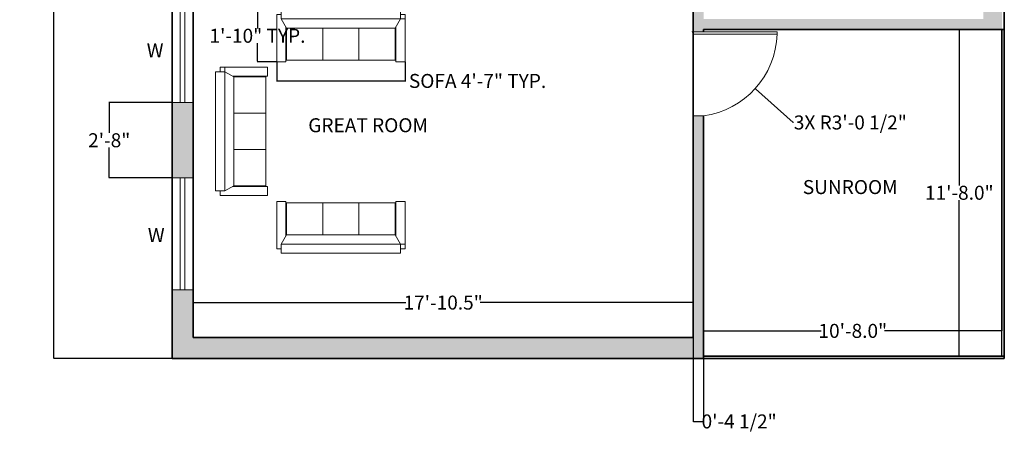
# Model space of a CAD drawing. Units: inches. Extents: x 302 to 1258, y 831 to 1373.
# Tile 7 of 13: x 781 to 1203, y 831 to 1012. Entities that reach past the tile are written whole.
import ezdxf

# ---------------------------------------------------------------- set-up
doc = ezdxf.new("R2010")
doc.units = ezdxf.units.IN
doc.header["$MEASUREMENT"] = 0
for name, color, linetype, lineweight in [('A-ANNO-DIMS', 2, 'Continuous', 18), ('A-ANNO-TEXT', 7, 'Continuous', 18), ('A-AREA-IDEN', 7, 'Continuous', 18), ('A-DOOR', 3, 'Continuous', 18), ('A-FURN', 8, 'Continuous', 18), ('A-GLAZ', 4, 'Continuous', 18), ('A-WALL', 7, 'Continuous', 35), ('A-WALL-PATT', 251, 'Continuous', 13)]:
    doc.layers.add(name, color=color, linetype=linetype, lineweight=lineweight)
doc.styles.get("Standard").update_dxf_attribs({"font": 'arial.ttf'})
doc.dimstyles.get("Standard").update_dxf_attribs({"dimtxt": 6, "dimasz": 0.18, "dimexe": 0.18, "dimexo": 0.0625, "dimgap": 0.09, "dimtad": 0, "dimtih": 1, "dimtoh": 1, "dimdec": 1, "dimzin": 0, "dimdsep": 46, "dimlunit": 3, "dimtxsty": 'Standard', "dimcen": 0.09, "dimadec": 0, "dimazin": 0, "dimtfac": 1, "dimtdec": 1, "dimtofl": 0, "dimtmove": 0, "dimatfit": 3, "dimfxl": 1, "dimtolj": 1, "dimtzin": 0, "dimarcsym": 0})

# ---------------------------------------------------------------- blocks, each defined once
blk = doc.blocks.new('*D27')
at = {"layer": 'A-ANNO-DIMS', "color": 0, "lineweight": -2, "transparency": 16777216}
for p, q in [((1074.12, 867.88), (1074.12, 878.8)), ((1202.12, 867.88), (1202.12, 878.8)), ((1074.3, 878.62), (1124.51, 878.62)), ((1201.94, 878.62), (1151.73, 878.62))]:
    blk.add_line(p, q, dxfattribs=at)
at = {"layer": 'A-ANNO-DIMS', "color": 0, "transparency": 16777216}
for points in [[(1074.3, 878.65), (1074.3, 878.59), (1074.12, 878.62)], [(1201.94, 878.65), (1201.94, 878.59), (1202.12, 878.62)]]:
    blk.add_solid(points, dxfattribs=at)
at = {"layer": 'Defpoints', "color": 0, "transparency": 16777216}
for p in [(1202.12, 878.62), (1074.12, 867.82), (1202.12, 867.82)]:
    blk.add_point(p, dxfattribs=at)
at = {"layer": 'A-ANNO-DIMS', "color": 0, "transparency": 16777216, "insert": (1138.12, 878.62), "char_height": 6, "attachment_point": 5}
blk.add_mtext('\\A1;10\'-8.0"', dxfattribs=at)
blk = doc.blocks.new('*D28')
at = {"layer": 'A-ANNO-DIMS', "color": 0, "lineweight": -2, "transparency": 16777216}
for p, q in [((1202.06, 1007.82), (1183.63, 1007.82)), ((1183.81, 1007.64), (1183.81, 940.97)), ((1183.81, 868), (1183.81, 934.67)), ((1202.06, 867.82), (1183.63, 867.82))]:
    blk.add_line(p, q, dxfattribs=at)
at = {"layer": 'A-ANNO-DIMS', "color": 0, "transparency": 16777216}
for points in [[(1183.78, 1007.64), (1183.84, 1007.64), (1183.81, 1007.82)], [(1183.78, 868), (1183.84, 868), (1183.81, 867.82)]]:
    blk.add_solid(points, dxfattribs=at)
at = {"layer": 'Defpoints', "color": 0, "transparency": 16777216}
for p in [(1202.12, 1007.82), (1183.81, 867.82), (1202.12, 867.82)]:
    blk.add_point(p, dxfattribs=at)
at = {"layer": 'A-ANNO-DIMS', "color": 0, "transparency": 16777216, "insert": (1183.81, 937.82), "char_height": 6, "attachment_point": 5}
blk.add_mtext('\\A1;11\'-8.0"', dxfattribs=at)
blk = doc.blocks.new('*D29')
at = {"layer": 'A-ANNO-DIMS', "color": 0, "lineweight": -2, "transparency": 16777216}
for p, q in [((855.12, 875.88), (855.12, 890.93)), ((855.3, 890.75), (946.43, 890.75)), ((1069.44, 890.75), (978.31, 890.75)), ((1069.62, 875.88), (1069.62, 890.93))]:
    blk.add_line(p, q, dxfattribs=at)
at = {"layer": 'A-ANNO-DIMS', "color": 0, "transparency": 16777216}
for points in [[(855.3, 890.78), (855.3, 890.72), (855.12, 890.75)], [(1069.44, 890.78), (1069.44, 890.72), (1069.62, 890.75)]]:
    blk.add_solid(points, dxfattribs=at)
at = {"layer": 'Defpoints', "color": 0, "transparency": 16777216}
for p in [(1069.62, 890.75), (855.12, 875.82), (1069.62, 875.82)]:
    blk.add_point(p, dxfattribs=at)
at = {"layer": 'A-ANNO-DIMS', "color": 0, "transparency": 16777216, "insert": (962.37, 890.75), "char_height": 6, "attachment_point": 5}
blk.add_mtext('\\A1;17\'-10.5"', dxfattribs=at)
blk = doc.blocks.new('*D34')
at = {"layer": 'A-ANNO-DIMS', "color": 0, "lineweight": -2, "transparency": 16777216}
for p, q in [((846.06, 1342.32), (795.24, 1342.32)), ((795.42, 1342.14), (795.42, 1107.72)), ((795.42, 867), (795.42, 1101.41)), ((846.06, 866.82), (795.24, 866.82))]:
    blk.add_line(p, q, dxfattribs=at)
at = {"layer": 'A-ANNO-DIMS', "color": 0, "transparency": 16777216}
for points in [[(795.39, 1342.14), (795.45, 1342.14), (795.42, 1342.32)], [(795.39, 867), (795.45, 867), (795.42, 866.82)]]:
    blk.add_solid(points, dxfattribs=at)
at = {"layer": 'Defpoints', "color": 0, "transparency": 16777216}
for p in [(846.12, 1342.32), (795.42, 866.82), (846.12, 866.82)]:
    blk.add_point(p, dxfattribs=at)
at = {"layer": 'A-ANNO-DIMS', "color": 0, "transparency": 16777216, "insert": (795.42, 1104.57), "char_height": 6, "attachment_point": 5}
blk.add_mtext('\\A1;39\'-7.5"', dxfattribs=at)
blk = doc.blocks.new('SOFA-3-SEAT')
for p, q in [((1.96, 55.04), (22.23, 55.04)), ((1.96, 55.04), (1.96, 53.08)), ((3.92, 55.04), (3.92, 1.96)), ((22.23, 51.12), (22.23, 55.04)), ((0, 53.08), (0, 1.96)), ((3.92, 53.08), (0, 53.08)), ((3.92, 53.08), (7.85, 50.88)), ((7.54, 51.12), (22.23, 51.12)), ((21.57, 50.87), (7.85, 50.87)), ((21.57, 35.3), (7.85, 35.3)), ((21.57, 19.74), (7.85, 19.74)), ((3.92, 1.96), (0, 1.96)), ((1.96, 1.96), (1.96, 0)), ((1.96, 0), (22.23, 0)), ((7.85, 4.17), (3.92, 1.96)), ((7.28, 3.92), (22.23, 3.92)), ((22.23, 3.92), (22.23, 0))]:
    blk.add_line(p, q)
blk.add_lwpolyline([(7.85, 50.88), (7.85, 4.17), (21.57, 4.17), (21.57, 50.87)])
blk = doc.blocks.new('WINDOW-48IN')
for p, q in [((0, 0), (0, 9)), ((0, 9), (48, 9)), ((48, 9), (48, 0)), ((0, 5.5), (48, 5.5)), ((48, 3.5), (0, 3.5)), ((48, 0), (0, 0))]:
    blk.add_line(p, q)
blk = doc.blocks.new('*D47')
at = {"layer": 'A-ANNO-DIMS', "color": 0, "lineweight": -2, "transparency": 16777216}
for p, q in [((890.97, 993.95), (890.97, 985.57)), ((946.01, 993.95), (946.01, 985.57)), ((891.15, 985.75), (945.83, 985.75)), ((946.01, 985.75), (946.19, 985.75))]:
    blk.add_line(p, q, dxfattribs=at)
at = {"layer": 'A-ANNO-DIMS', "color": 0, "transparency": 16777216}
for points in [[(891.15, 985.78), (891.15, 985.72), (890.97, 985.75)], [(945.83, 985.78), (945.83, 985.72), (946.01, 985.75)]]:
    blk.add_solid(points, dxfattribs=at)
at = {"layer": 'Defpoints', "color": 0, "transparency": 16777216}
for p in [(890.97, 994.01), (946.01, 994.01), (946.01, 985.75)]:
    blk.add_point(p, dxfattribs=at)
at = {"layer": 'A-ANNO-DIMS', "color": 0, "transparency": 16777216, "insert": (977.13, 985.75), "char_height": 6, "attachment_point": 5}
blk.add_mtext('\\A1;SOFA 4\'-7" TYP.', dxfattribs=at)
blk = doc.blocks.new('*D48')
at = {"layer": 'A-ANNO-DIMS', "color": 0, "lineweight": -2, "transparency": 16777216}
for p, q in [((890.9, 1016.24), (882.53, 1016.24)), ((882.71, 1016.06), (882.71, 1008.28)), ((882.71, 994.19), (882.71, 1001.97)), ((890.9, 994.01), (882.53, 994.01))]:
    blk.add_line(p, q, dxfattribs=at)
at = {"layer": 'A-ANNO-DIMS', "color": 0, "transparency": 16777216}
for points in [[(882.68, 1016.06), (882.74, 1016.06), (882.71, 1016.24)], [(882.68, 994.19), (882.74, 994.19), (882.71, 994.01)]]:
    blk.add_solid(points, dxfattribs=at)
at = {"layer": 'Defpoints', "color": 0, "transparency": 16777216}
for p in [(890.97, 1016.24), (882.71, 994.01), (890.97, 994.01)]:
    blk.add_point(p, dxfattribs=at)
at = {"layer": 'A-ANNO-DIMS', "color": 0, "transparency": 16777216, "insert": (882.71, 1005.12), "char_height": 6, "attachment_point": 5}
blk.add_mtext('\\A1;1\'-10" TYP.', dxfattribs=at)
blk = doc.blocks.new('*D84')
at = {"layer": 'A-ANNO-DIMS', "color": 0, "lineweight": -2, "transparency": 16777216}
for p, q in [((1069.62, 875.76), (1069.62, 839.64)), ((1074.12, 866.76), (1074.12, 839.64)), ((1069.8, 839.82), (1073.94, 839.82)), ((1074.12, 839.82), (1074.3, 839.82))]:
    blk.add_line(p, q, dxfattribs=at)
at = {"layer": 'A-ANNO-DIMS', "color": 0, "transparency": 16777216}
for points in [[(1069.8, 839.85), (1069.8, 839.79), (1069.62, 839.82)], [(1073.94, 839.85), (1073.94, 839.79), (1074.12, 839.82)]]:
    blk.add_solid(points, dxfattribs=at)
at = {"layer": 'Defpoints', "color": 0, "transparency": 16777216}
for p in [(1069.62, 875.82), (1074.12, 866.82), (1074.12, 839.82)]:
    blk.add_point(p, dxfattribs=at)
at = {"layer": 'A-ANNO-DIMS', "color": 0, "transparency": 16777216, "insert": (1089.36, 839.82), "char_height": 6, "attachment_point": 5}
blk.add_mtext('\\A1;0\'-4 1/2"', dxfattribs=at)
blk = doc.blocks.new('*D90')
at = {"layer": 'A-ANNO-DIMS', "color": 0, "lineweight": -2, "transparency": 16777216}
for p, q in [((846.06, 976.44), (818.94, 976.44)), ((819.12, 976.26), (819.12, 963.47)), ((819.12, 944.38), (819.12, 957.17)), ((846.06, 944.2), (818.94, 944.2))]:
    blk.add_line(p, q, dxfattribs=at)
at = {"layer": 'A-ANNO-DIMS', "color": 0, "transparency": 16777216}
for points in [[(819.09, 976.26), (819.15, 976.26), (819.12, 976.44)], [(819.09, 944.38), (819.15, 944.38), (819.12, 944.2)]]:
    blk.add_solid(points, dxfattribs=at)
at = {"layer": 'Defpoints', "color": 0, "transparency": 16777216}
for p in [(846.12, 976.44), (819.12, 944.2), (846.12, 944.2)]:
    blk.add_point(p, dxfattribs=at)
at = {"layer": 'A-ANNO-DIMS', "color": 0, "transparency": 16777216, "insert": (819.12, 960.32), "char_height": 6, "attachment_point": 5}
blk.add_mtext('\\A1;2\'-8"', dxfattribs=at)
blk = doc.blocks.new('*D96')
at = {"layer": 'A-ANNO-DIMS', "color": 0, "lineweight": -2, "transparency": 16777216}
for p, q in [((1069.21, 1006.82), (1069.39, 1006.82)), ((1069.3, 1006.73), (1069.3, 1006.91)), ((1112.5, 967.95), (1096.44, 982.41)), ((1112.68, 967.95), (1112.5, 967.95))]:
    blk.add_line(p, q, dxfattribs=at)
at = {"layer": 'A-ANNO-DIMS', "color": 0, "transparency": 16777216}
blk.add_solid([(1096.46, 982.43), (1096.42, 982.38), (1096.3, 982.53)], dxfattribs=at)
at = {"layer": 'Defpoints', "color": 0, "transparency": 16777216}
for p in [(1069.3, 1006.82), (1096.3, 982.53)]:
    blk.add_point(p, dxfattribs=at)
at = {"layer": 'A-ANNO-DIMS', "color": 0, "transparency": 16777216, "insert": (1137.06, 967.95), "char_height": 6, "attachment_point": 5}
blk.add_mtext('\\A1;3X R3\'-0 1/2"', dxfattribs=at)

msp = doc.modelspace()

# ---------------------------------------------------------------- hatches: boundary and pattern name
at = {"layer": 'A-WALL-PATT'}
h = msp.add_hatch(color=256, dxfattribs=at)
h.dxf.hatch_style = 1
h.paths.add_polyline_path([(1003.23, 1342.32), (934.03, 1342.32), (934.03, 1333.32), (975.12, 1333.32), (975.12, 1330.32), (979.62, 1330.32), (979.62, 1333.32), (1003.23, 1333.32)])
h.paths.add_polyline_path([(1203.12, 1342.32), (1027.23, 1342.32), (1027.23, 1333.32), (1045.62, 1333.32), (1045.62, 1213.32), (979.62, 1213.32), (979.62, 1306.32), (975.12, 1306.32), (975.12, 1213.32), (974.12, 1213.32), (974.12, 1208.82), (975.12, 1208.82), (1051.12, 1208.82), (1051.12, 1213.32), (1050.12, 1213.32), (1050.12, 1333.32), (1194.12, 1333.32), (1194.12, 1302.71), (1203.12, 1302.71)])
h.paths.add_polyline_path([(855.12, 1333.32), (886.03, 1333.32), (886.03, 1342.32), (846.12, 1342.32), (846.12, 1300.76), (855.12, 1300.76)])
h.paths.add_polyline_path([(938.12, 1213.32), (855.12, 1213.32), (855.12, 1252.76), (846.12, 1252.76), (846.12, 1164.55), (855.12, 1164.55), (855.12, 1208.82), (933.12, 1208.82), (933.12, 1082.82), (937.62, 1082.82), (937.62, 1208.82), (938.12, 1208.82)])
h.paths.add_polyline_path([(855.12, 1116.55), (846.12, 1116.55), (846.12, 1024.44), (855.12, 1024.44)])
h.paths.add_polyline_path([(855.12, 976.44), (846.12, 976.44), (846.12, 944.2), (855.12, 944.2)])
h = msp.add_hatch(color=256, dxfattribs=at)
h.dxf.hatch_style = 1
h.paths.add_polyline_path([(1074.12, 970.82), (1069.62, 970.82), (1069.62, 875.82), (855.12, 875.82), (855.12, 896.2), (846.12, 896.2), (846.12, 866.82), (1074.12, 866.82)])
h.paths.add_polyline_path([(1202.12, 1049.42), (1194.12, 1049.42), (1194.12, 1012.32), (1074.12, 1012.32), (1074.12, 1093.32), (1069.62, 1093.32), (1069.62, 1006.82), (1074.12, 1006.82), (1074.12, 1007.82), (1194.12, 1007.82), (1202.12, 1007.82)])

# ---------------------------------------------------------------- linework, layer by layer
at = {"layer": 'A-DOOR'}
for p, q in [((1069.62, 1007.82), (1069.62, 1006.82)), ((1069.62, 1006.82), (1105.62, 1006.82)), ((1069.62, 1006.82), (1069.62, 970.82)), ((1105.62, 1005.82), (1069.62, 1005.82)), ((1105.62, 1006.82), (1105.62, 1005.82)), ((1069.62, 970.82), (1074.12, 970.82))]:
    msp.add_line(p, q, dxfattribs=at)
msp.add_arc((1069.3, 1006.82), 36.32, 277.6281, 358.4223, dxfattribs=at)
at = {"layer": 'A-WALL'}
for p, q in [((846.12, 1342.32), (846.12, 866.82)), ((1203.12, 866.82), (1203.12, 1342.32)), ((855.12, 1208.82), (855.12, 875.82)), ((1069.62, 1136.82), (1069.62, 875.82)), ((1203.12, 1097.42), (1203.12, 866.82)), ((1074.12, 1007.82), (1194.12, 1007.82)), ((1074.12, 1007.82), (1074.12, 1006.82)), ((1194.12, 1007.82), (1202.12, 1007.82)), ((1202.12, 1007.82), (1203.12, 1007.82)), ((1202.12, 878.62), (1202.12, 1007.82)), ((1074.12, 970.82), (1074.12, 866.82)), ((855.12, 875.82), (1069.62, 875.82)), ((846.12, 866.82), (1203.12, 866.82)), ((1074.12, 867.82), (1203.12, 867.82))]:
    msp.add_line(p, q, dxfattribs=at)

# ---------------------------------------------------------------- block references
at = {"layer": 'A-FURN', "rotation": 269.9999999999992}
msp.add_blockref('SOFA-3-SEAT', (890.97, 1016.24), dxfattribs=at)
at = {"layer": 'A-FURN'}
msp.add_blockref('SOFA-3-SEAT', (864.75, 936.64), dxfattribs=at)
at = {"layer": 'A-FURN', "extrusion": (0, 0, -1), "zscale": -1, "rotation": 90.00000000000014}
msp.add_blockref('SOFA-3-SEAT', (-890.97, 911.89), dxfattribs=at)
at = {"layer": 'A-GLAZ'}
for p, rotation in [((855.12, 976.44), 89.99999999999999), ((855.12, 896.2), 89.99999999999952)]:
    msp.add_blockref('WINDOW-48IN', p, dxfattribs=dict(at, rotation=rotation))

# ---------------------------------------------------------------- texts
at = {"layer": 'A-ANNO-TEXT', "char_height": 6, "attachment_point": 1}
for insert in [(835.21, 1001.86), (835.68, 922.67)]:
    msp.add_mtext_dynamic_manual_height_columns('W', width=16.4894, gutter_width=30, heights=[0], dxfattribs=dict(at, insert=insert))
at = {"layer": 'A-AREA-IDEN', "char_height": 6, "attachment_point": 1}
for s, width, insert in [('GREAT ROOM', 95.2258, (904.51, 969.76)), ('SUNROOM', 53.6425, (1116.68, 943.26))]:
    msp.add_mtext_dynamic_manual_height_columns(s, width=width, gutter_width=30, heights=[0], dxfattribs=dict(at, insert=insert))

# ---------------------------------------------------------------- dimensions: what is measured, and where the dimension line sits
at = {"layer": 'A-ANNO-DIMS'}
for base, p1, p2, override, picture, middle in [((795.42, 866.82), (846.12, 1342.32), (846.12, 866.82), {"dimclrd": 0, "dimclre": 0, "dimclrt": 0}, '*D34', (795.42, 1104.57)), ((1183.81, 867.82), (1202.12, 1007.82), (1202.12, 867.82), {"dimclrd": 0, "dimclre": 0, "dimclrt": 0}, '*D28', (1183.81, 937.82)), ((819.12, 944.2), (846.12, 976.44), (846.12, 944.2), {"dimdec": 1, "dimlfac": 1, "dimrnd": 0, "dimzin": 1, "dimdsep": 46, "dimlunit": 4, "dimfrac": 2}, '*D90', (819.12, 960.32))]:
    dim = msp.add_linear_dim(base=base, p1=p1, p2=p2, angle=90, dimstyle='Standard', override=override, dxfattribs=at)
    dim.commit()
    dim.dimension.update_dxf_attribs({"geometry": picture, "text_midpoint": middle})
dim = msp.add_linear_dim(base=(882.71, 994.01), p1=(890.97, 1016.24), p2=(890.97, 994.01), angle=270, text='<> TYP.', dimstyle='Standard', override={"dimdec": 1, "dimlfac": 1, "dimrnd": 0, "dimzin": 1, "dimdsep": 46, "dimlunit": 4, "dimfrac": 2}, dxfattribs=at)
dim.commit()
dim.dimension.update_dxf_attribs({"geometry": '*D48', "text_midpoint": (882.71, 1005.12)})
dim = msp.add_radius_dim(center=(1069.3, 1006.82), mpoint=(1096.3, 982.53), text='3X <>', dimstyle='Standard', override={"dimdec": 1, "dimlfac": 1, "dimrnd": 0, "dimzin": 1, "dimdsep": 46, "dimlunit": 4, "dimfrac": 2}, dxfattribs=at)
dim.commit()
dim.dimension.update_dxf_attribs({"geometry": '*D96', "text_midpoint": (1137.06, 967.95), "dimtype": 164})
dim = msp.add_linear_dim(base=(946.01, 985.75), p1=(890.97, 994.01), p2=(946.01, 994.01), text='SOFA <> TYP.', dimstyle='Standard', override={"dimdec": 1, "dimlfac": 1, "dimrnd": 0, "dimzin": 1, "dimdsep": 46, "dimlunit": 4, "dimfrac": 2}, dxfattribs=at)
dim.commit()
dim.dimension.update_dxf_attribs({"geometry": '*D47', "text_midpoint": (977.13, 985.75)})
for base, p1, p2, override, picture, middle in [((1069.62, 890.75), (855.12, 875.82), (1069.62, 875.82), {"dimclrd": 0, "dimclre": 0, "dimclrt": 0}, '*D29', (962.37, 890.75)), ((1202.12, 878.62), (1074.12, 867.82), (1202.12, 867.82), {"dimclrd": 0, "dimclre": 0, "dimclrt": 0}, '*D27', (1138.12, 878.62)), ((1074.12, 839.82), (1069.62, 875.82), (1074.12, 866.82), {"dimdec": 1, "dimlfac": 1, "dimrnd": 0, "dimzin": 1, "dimdsep": 46, "dimlunit": 4, "dimfrac": 2}, '*D84', (1089.36, 839.82))]:
    dim = msp.add_linear_dim(base=base, p1=p1, p2=p2, dimstyle='Standard', override=override, dxfattribs=at)
    dim.commit()
    dim.dimension.update_dxf_attribs({"geometry": picture, "text_midpoint": middle})

doc.saveas('drawing.dxf')
